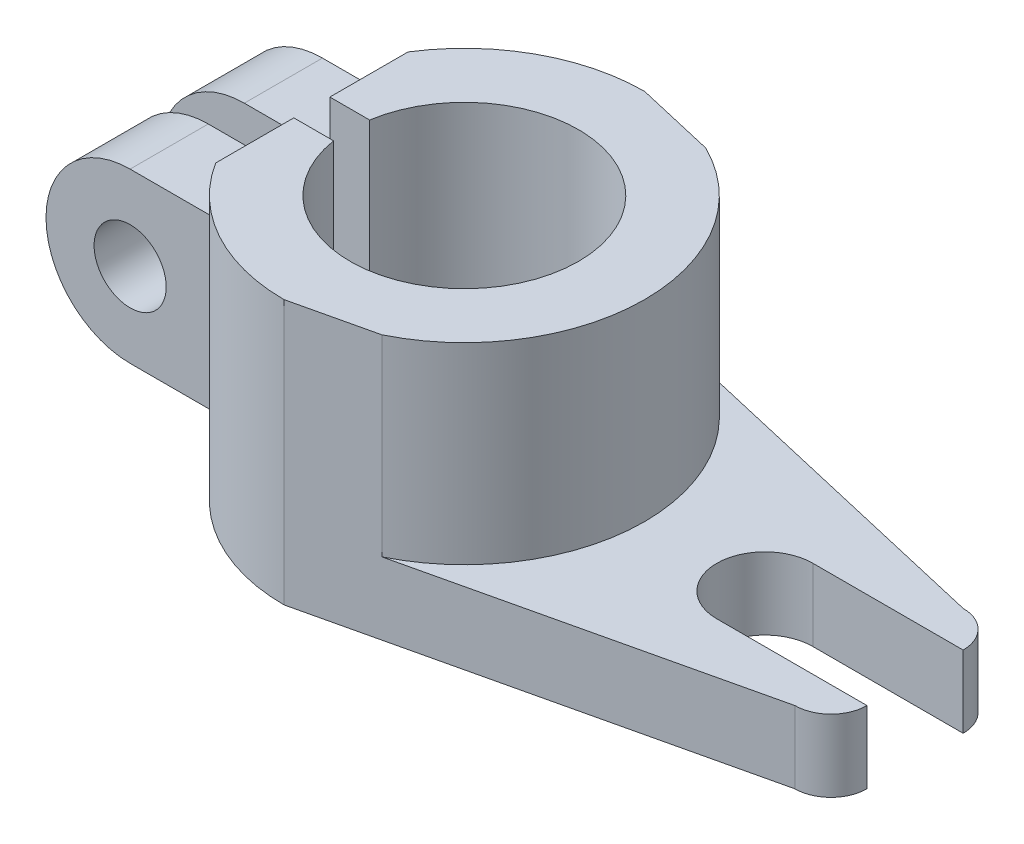
ISO-10303-21;
HEADER;
FILE_DESCRIPTION(('STEP AP214'),'2;1');
FILE_NAME('part.step','',(''),(''),'','','');
FILE_SCHEMA(('AUTOMOTIVE_DESIGN { 1 0 10303 214 1 1 1 1 }'));
ENDSEC;
DATA;
#1=APPLICATION_CONTEXT('core data for automotive mechanical design processes');
#2=APPLICATION_PROTOCOL_DEFINITION('international standard','automotive_design',2000,#1);
#3=PRODUCT_CONTEXT('',#1,'mechanical');
#4=PRODUCT('Part','Part','',(#3));
#5=PRODUCT_RELATED_PRODUCT_CATEGORY('part','',(#4));
#6=PRODUCT_DEFINITION_FORMATION('','',#4);
#7=PRODUCT_DEFINITION_CONTEXT('part definition',#1,'design');
#8=PRODUCT_DEFINITION('design','',#6,#7);
#9=PRODUCT_DEFINITION_SHAPE('','',#8);
#10=(LENGTH_UNIT() NAMED_UNIT(*) SI_UNIT(.MILLI.,.METRE.));
#11=(NAMED_UNIT(*) PLANE_ANGLE_UNIT() SI_UNIT($,.RADIAN.));
#12=(NAMED_UNIT(*) SI_UNIT($,.STERADIAN.) SOLID_ANGLE_UNIT());
#13=UNCERTAINTY_MEASURE_WITH_UNIT(LENGTH_MEASURE(1.E-05),#10,'distance_accuracy_value','');
#14=(GEOMETRIC_REPRESENTATION_CONTEXT(3) GLOBAL_UNCERTAINTY_ASSIGNED_CONTEXT((#13)) GLOBAL_UNIT_ASSIGNED_CONTEXT((#10,
#11,#12)) REPRESENTATION_CONTEXT('',''));
#15=CARTESIAN_POINT('',(0.,0.,0.));
#16=DIRECTION('',(0.,0.,1.));
#17=DIRECTION('',(1.,0.,0.));
#18=AXIS2_PLACEMENT_3D('',#15,#16,#17);
#19=CARTESIAN_POINT('',(-39.6122656575528,22.,-16.));
#20=DIRECTION('',(0.,0.,1.));
#21=DIRECTION('',(1.,0.,0.));
#22=AXIS2_PLACEMENT_3D('',#19,#20,#21);
#23=CYLINDRICAL_SURFACE('',#22,14.);
#24=DIRECTION('',(0.,0.,1.));
#25=VECTOR('',#24,1.);
#26=CARTESIAN_POINT('',(-39.6122656575528,36.,-16.));
#27=LINE('',#26,#25);
#28=CARTESIAN_POINT('',(-39.6122656575528,36.,3.));
#29=VERTEX_POINT('',#28);
#30=CARTESIAN_POINT('',(-39.6122656575528,36.,16.));
#31=VERTEX_POINT('',#30);
#32=EDGE_CURVE('E333',#29,#31,#27,.T.);
#33=ORIENTED_EDGE('',*,*,#32,.F.);
#34=CARTESIAN_POINT('',(-39.6122656575528,22.,3.));
#35=DIRECTION('',(0.,0.,1.));
#36=DIRECTION('',(1.,0.,0.));
#37=AXIS2_PLACEMENT_3D('',#34,#35,#36);
#38=CIRCLE('',#37,14.);
#39=CARTESIAN_POINT('',(-39.6122656575528,8.,3.));
#40=VERTEX_POINT('',#39);
#41=EDGE_CURVE('E56',#40,#29,#38,.F.);
#42=ORIENTED_EDGE('',*,*,#41,.F.);
#43=DIRECTION('',(0.,0.,1.));
#44=VECTOR('',#43,1.);
#45=CARTESIAN_POINT('',(-39.6122656575528,8.,-16.));
#46=LINE('',#45,#44);
#47=CARTESIAN_POINT('',(-39.6122656575528,8.,16.));
#48=VERTEX_POINT('',#47);
#49=EDGE_CURVE('E336',#40,#48,#46,.T.);
#50=ORIENTED_EDGE('',*,*,#49,.T.);
#51=CARTESIAN_POINT('',(-39.6122656575528,22.,16.));
#52=DIRECTION('',(0.,0.,1.));
#53=DIRECTION('',(1.,0.,0.));
#54=AXIS2_PLACEMENT_3D('',#51,#52,#53);
#55=CIRCLE('',#54,14.);
#56=EDGE_CURVE('E329',#31,#48,#55,.T.);
#57=ORIENTED_EDGE('',*,*,#56,.F.);
#58=EDGE_LOOP('',(#33,#42,#50,#57));
#59=FACE_BOUND('',#58,.T.);
#60=ADVANCED_FACE('F43',(#59),#23,.T.);
#61=CARTESIAN_POINT('',(-39.6122656575528,22.,-3.));
#62=DIRECTION('',(0.,0.,1.));
#63=DIRECTION('',(1.,0.,0.));
#64=AXIS2_PLACEMENT_3D('',#61,#62,#63);
#65=CIRCLE('',#64,14.);
#66=CARTESIAN_POINT('',(-39.6122656575528,8.,-3.));
#67=VERTEX_POINT('',#66);
#68=CARTESIAN_POINT('',(-39.6122656575528,36.,-3.));
#69=VERTEX_POINT('',#68);
#70=EDGE_CURVE('E453',#67,#69,#65,.F.);
#71=ORIENTED_EDGE('',*,*,#70,.T.);
#72=CARTESIAN_POINT('',(-39.6122656575528,36.,-16.));
#73=VERTEX_POINT('',#72);
#74=EDGE_CURVE('E294',#73,#69,#27,.T.);
#75=ORIENTED_EDGE('',*,*,#74,.F.);
#76=CARTESIAN_POINT('',(-39.6122656575528,22.,-16.));
#77=DIRECTION('',(0.,0.,1.));
#78=DIRECTION('',(1.,0.,0.));
#79=AXIS2_PLACEMENT_3D('',#76,#77,#78);
#80=CIRCLE('',#79,14.);
#81=CARTESIAN_POINT('',(-39.6122656575528,8.,-16.));
#82=VERTEX_POINT('',#81);
#83=EDGE_CURVE('E326',#73,#82,#80,.T.);
#84=ORIENTED_EDGE('',*,*,#83,.T.);
#85=EDGE_CURVE('E332',#82,#67,#46,.T.);
#86=ORIENTED_EDGE('',*,*,#85,.T.);
#87=EDGE_LOOP('',(#71,#75,#84,#86));
#88=FACE_BOUND('',#87,.T.);
#89=ADVANCED_FACE('F460',(#88),#23,.T.);
#90=CARTESIAN_POINT('',(-39.6122656575528,22.,-22.0274259538665));
#91=DIRECTION('',(0.,0.,1.));
#92=DIRECTION('',(1.,0.,0.));
#93=AXIS2_PLACEMENT_3D('',#90,#91,#92);
#94=CYLINDRICAL_SURFACE('',#93,6.);
#95=CARTESIAN_POINT('',(-39.6122656575528,22.,-16.));
#96=DIRECTION('',(0.,0.,-1.));
#97=DIRECTION('',(-1.,0.,0.));
#98=AXIS2_PLACEMENT_3D('',#95,#96,#97);
#99=CIRCLE('',#98,6.);
#100=CARTESIAN_POINT('',(-45.6122656575528,22.,-16.));
#101=VERTEX_POINT('',#100);
#102=EDGE_CURVE('E50',#101,#101,#99,.T.);
#103=ORIENTED_EDGE('',*,*,#102,.T.);
#104=EDGE_LOOP('',(#103));
#105=FACE_BOUND('',#104,.T.);
#106=CARTESIAN_POINT('',(-39.6122656575528,22.,-3.));
#107=DIRECTION('',(0.,0.,1.));
#108=DIRECTION('',(1.,0.,0.));
#109=AXIS2_PLACEMENT_3D('',#106,#107,#108);
#110=CIRCLE('',#109,6.);
#111=CARTESIAN_POINT('',(-33.6122656575528,22.,-3.));
#112=VERTEX_POINT('',#111);
#113=EDGE_CURVE('E454',#112,#112,#110,.F.);
#114=ORIENTED_EDGE('',*,*,#113,.F.);
#115=EDGE_LOOP('',(#114));
#116=FACE_BOUND('',#115,.T.);
#117=ADVANCED_FACE('F476',(#105,#116),#94,.F.);
#118=CARTESIAN_POINT('',(0.,8.,-16.));
#119=DIRECTION('',(0.,1.,0.));
#120=DIRECTION('',(0.,0.,1.));
#121=AXIS2_PLACEMENT_3D('',#118,#119,#120);
#122=PLANE('',#121);
#123=DIRECTION('',(1.,0.,0.));
#124=VECTOR('',#123,1.);
#125=CARTESIAN_POINT('',(0.,8.,-3.));
#126=LINE('',#125,#124);
#127=CARTESIAN_POINT('',(-25.377155080899,8.,-3.));
#128=VERTEX_POINT('',#127);
#129=EDGE_CURVE('E296',#67,#128,#126,.T.);
#130=ORIENTED_EDGE('',*,*,#129,.F.);
#131=ORIENTED_EDGE('',*,*,#85,.F.);
#132=DIRECTION('',(-1.,0.,0.));
#133=VECTOR('',#132,1.);
#134=CARTESIAN_POINT('',(0.,8.,-16.));
#135=LINE('',#134,#133);
#136=CARTESIAN_POINT('',(-25.377155080899,8.,-16.));
#137=VERTEX_POINT('',#136);
#138=EDGE_CURVE('E422',#137,#82,#135,.T.);
#139=ORIENTED_EDGE('',*,*,#138,.F.);
#140=DIRECTION('',(0.,0.,1.));
#141=VECTOR('',#140,1.);
#142=CARTESIAN_POINT('',(-25.377155080899,8.,-16.));
#143=LINE('',#142,#141);
#144=EDGE_CURVE('E424',#137,#128,#143,.T.);
#145=ORIENTED_EDGE('',*,*,#144,.T.);
#146=EDGE_LOOP('',(#130,#131,#139,#145));
#147=FACE_BOUND('',#146,.T.);
#148=ADVANCED_FACE('F463',(#147),#122,.F.);
#149=CARTESIAN_POINT('',(0.,36.,-16.));
#150=DIRECTION('',(0.,-1.,0.));
#151=DIRECTION('',(0.,0.,-1.));
#152=AXIS2_PLACEMENT_3D('',#149,#150,#151);
#153=PLANE('',#152);
#154=DIRECTION('',(-1.,0.,0.));
#155=VECTOR('',#154,1.);
#156=CARTESIAN_POINT('',(0.,36.,-3.));
#157=LINE('',#156,#155);
#158=CARTESIAN_POINT('',(-25.377155080899,36.,-3.));
#159=VERTEX_POINT('',#158);
#160=EDGE_CURVE('E286',#159,#69,#157,.T.);
#161=ORIENTED_EDGE('',*,*,#160,.F.);
#162=DIRECTION('',(0.,0.,1.));
#163=VECTOR('',#162,1.);
#164=CARTESIAN_POINT('',(-25.377155080899,36.,-16.));
#165=LINE('',#164,#163);
#166=CARTESIAN_POINT('',(-25.377155080899,36.,-16.));
#167=VERTEX_POINT('',#166);
#168=EDGE_CURVE('E292',#167,#159,#165,.T.);
#169=ORIENTED_EDGE('',*,*,#168,.F.);
#170=DIRECTION('',(1.,0.,0.));
#171=VECTOR('',#170,1.);
#172=CARTESIAN_POINT('',(0.,36.,-16.));
#173=LINE('',#172,#171);
#174=EDGE_CURVE('E443',#73,#167,#173,.T.);
#175=ORIENTED_EDGE('',*,*,#174,.F.);
#176=ORIENTED_EDGE('',*,*,#74,.T.);
#177=EDGE_LOOP('',(#161,#169,#175,#176));
#178=FACE_BOUND('',#177,.T.);
#179=ADVANCED_FACE('F289',(#178),#153,.F.);
#180=CARTESIAN_POINT('',(0.,44.,16.));
#181=DIRECTION('',(0.,0.,-1.));
#182=DIRECTION('',(-1.,0.,0.));
#183=AXIS2_PLACEMENT_3D('',#180,#181,#182);
#184=PLANE('',#183);
#185=CARTESIAN_POINT('',(-39.6122656575528,22.,16.));
#186=DIRECTION('',(0.,0.,1.));
#187=DIRECTION('',(1.,0.,0.));
#188=AXIS2_PLACEMENT_3D('',#185,#186,#187);
#189=CIRCLE('',#188,6.);
#190=CARTESIAN_POINT('',(-33.6122656575528,22.,16.));
#191=VERTEX_POINT('',#190);
#192=EDGE_CURVE('E340',#191,#191,#189,.T.);
#193=ORIENTED_EDGE('',*,*,#192,.F.);
#194=EDGE_LOOP('',(#193));
#195=FACE_BOUND('',#194,.T.);
#196=DIRECTION('',(1.,0.,0.));
#197=VECTOR('',#196,1.);
#198=CARTESIAN_POINT('',(0.,36.,16.));
#199=LINE('',#198,#197);
#200=CARTESIAN_POINT('',(-25.377155080899,36.,16.));
#201=VERTEX_POINT('',#200);
#202=EDGE_CURVE('E430',#31,#201,#199,.T.);
#203=ORIENTED_EDGE('',*,*,#202,.F.);
#204=ORIENTED_EDGE('',*,*,#56,.T.);
#205=DIRECTION('',(-1.,0.,0.));
#206=VECTOR('',#205,1.);
#207=CARTESIAN_POINT('',(0.,8.,16.));
#208=LINE('',#207,#206);
#209=CARTESIAN_POINT('',(-25.377155080899,8.,16.));
#210=VERTEX_POINT('',#209);
#211=EDGE_CURVE('E414',#210,#48,#208,.T.);
#212=ORIENTED_EDGE('',*,*,#211,.F.);
#213=DIRECTION('',(0.,-1.,0.));
#214=VECTOR('',#213,1.);
#215=CARTESIAN_POINT('',(-25.377155080899,44.,16.));
#216=LINE('',#215,#214);
#217=EDGE_CURVE('E345',#201,#210,#216,.T.);
#218=ORIENTED_EDGE('',*,*,#217,.F.);
#219=EDGE_LOOP('',(#203,#204,#212,#218));
#220=FACE_BOUND('',#219,.T.);
#221=ADVANCED_FACE('F482',(#195,#220),#184,.F.);
#222=CARTESIAN_POINT('',(0.,44.,-16.));
#223=DIRECTION('',(0.,0.,-1.));
#224=DIRECTION('',(-1.,0.,0.));
#225=AXIS2_PLACEMENT_3D('',#222,#223,#224);
#226=PLANE('',#225);
#227=ORIENTED_EDGE('',*,*,#102,.F.);
#228=EDGE_LOOP('',(#227));
#229=FACE_BOUND('',#228,.T.);
#230=ORIENTED_EDGE('',*,*,#83,.F.);
#231=ORIENTED_EDGE('',*,*,#174,.T.);
#232=DIRECTION('',(0.,-1.,0.));
#233=VECTOR('',#232,1.);
#234=CARTESIAN_POINT('',(-25.377155080899,44.,-16.));
#235=LINE('',#234,#233);
#236=EDGE_CURVE('E343',#167,#137,#235,.T.);
#237=ORIENTED_EDGE('',*,*,#236,.T.);
#238=ORIENTED_EDGE('',*,*,#138,.T.);
#239=EDGE_LOOP('',(#230,#231,#237,#238));
#240=FACE_BOUND('',#239,.T.);
#241=ADVANCED_FACE('F485',(#229,#240),#226,.T.);
#242=CARTESIAN_POINT('',(0.,44.,0.));
#243=DIRECTION('',(0.,-1.,0.));
#244=DIRECTION('',(0.,0.,-1.));
#245=AXIS2_PLACEMENT_3D('',#242,#243,#244);
#246=CYLINDRICAL_SURFACE('',#245,30.);
#247=CARTESIAN_POINT('',(-25.377155080899,44.,16.));
#248=VERTEX_POINT('',#247);
#249=EDGE_CURVE('E342',#248,#201,#216,.T.);
#250=ORIENTED_EDGE('',*,*,#249,.T.);
#251=ORIENTED_EDGE('',*,*,#217,.T.);
#252=DIRECTION('',(0.,1.,0.));
#253=VECTOR('',#252,1.);
#254=CARTESIAN_POINT('',(-25.377155080899,0.,16.));
#255=LINE('',#254,#253);
#256=CARTESIAN_POINT('',(-25.377155080899,0.,16.));
#257=VERTEX_POINT('',#256);
#258=EDGE_CURVE('E410',#257,#210,#255,.T.);
#259=ORIENTED_EDGE('',*,*,#258,.F.);
#260=CARTESIAN_POINT('',(0.,0.,0.));
#261=DIRECTION('',(0.,1.,0.));
#262=DIRECTION('',(0.,0.,1.));
#263=AXIS2_PLACEMENT_3D('',#260,#261,#262);
#264=CIRCLE('',#263,30.);
#265=CARTESIAN_POINT('',(0.,0.,30.));
#266=VERTEX_POINT('',#265);
#267=EDGE_CURVE('E351',#257,#266,#264,.T.);
#268=ORIENTED_EDGE('',*,*,#267,.T.);
#269=DIRECTION('',(0.,-1.,0.));
#270=VECTOR('',#269,1.);
#271=CARTESIAN_POINT('',(0.,44.,30.));
#272=LINE('',#271,#270);
#273=CARTESIAN_POINT('',(0.,44.,30.));
#274=VERTEX_POINT('',#273);
#275=EDGE_CURVE('E367',#274,#266,#272,.T.);
#276=ORIENTED_EDGE('',*,*,#275,.F.);
#277=CARTESIAN_POINT('',(0.,44.,0.));
#278=DIRECTION('',(0.,1.,0.));
#279=DIRECTION('',(0.,0.,1.));
#280=AXIS2_PLACEMENT_3D('',#277,#278,#279);
#281=CIRCLE('',#280,30.);
#282=EDGE_CURVE('E370',#248,#274,#281,.T.);
#283=ORIENTED_EDGE('',*,*,#282,.F.);
#284=EDGE_LOOP('',(#250,#251,#259,#268,#276,#283));
#285=FACE_BOUND('',#284,.T.);
#286=ADVANCED_FACE('F404',(#285),#246,.T.);
#287=CARTESIAN_POINT('',(6.60155471397249,12.,28.4692047040064));
#288=DIRECTION('',(-0.225890482018287,0.,-0.974152703703863));
#289=DIRECTION('',(-0.974152703703863,0.,0.225890482018287));
#290=AXIS2_PLACEMENT_3D('',#287,#288,#289);
#291=PLANE('',#290);
#292=DIRECTION('',(0.974152703703863,0.,-0.225890482018287));
#293=VECTOR('',#292,1.);
#294=CARTESIAN_POINT('',(6.60155471397249,0.,28.4692047040064));
#295=LINE('',#294,#293);
#296=CARTESIAN_POINT('',(69.,0.,14.));
#297=VERTEX_POINT('',#296);
#298=EDGE_CURVE('E144',#266,#297,#295,.T.);
#299=ORIENTED_EDGE('',*,*,#298,.T.);
#300=DIRECTION('',(0.,-1.,0.));
#301=VECTOR('',#300,1.);
#302=CARTESIAN_POINT('',(69.,12.,14.));
#303=LINE('',#302,#301);
#304=CARTESIAN_POINT('',(69.,12.,14.));
#305=VERTEX_POINT('',#304);
#306=EDGE_CURVE('E11',#305,#297,#303,.T.);
#307=ORIENTED_EDGE('',*,*,#306,.F.);
#308=DIRECTION('',(0.974152703703863,0.,-0.225890482018287));
#309=VECTOR('',#308,1.);
#310=CARTESIAN_POINT('',(6.60155471397249,12.,28.4692047040064));
#311=LINE('',#310,#309);
#312=CARTESIAN_POINT('',(13.2031094279449,12.,26.9384094080128));
#313=VERTEX_POINT('',#312);
#314=EDGE_CURVE('E105',#313,#305,#311,.T.);
#315=ORIENTED_EDGE('',*,*,#314,.F.);
#316=DIRECTION('',(0.,-1.,0.));
#317=VECTOR('',#316,1.);
#318=CARTESIAN_POINT('',(13.2031094279449,44.,26.9384094080128));
#319=LINE('',#318,#317);
#320=CARTESIAN_POINT('',(13.2031094279449,44.,26.9384094080128));
#321=VERTEX_POINT('',#320);
#322=EDGE_CURVE('E150',#321,#313,#319,.T.);
#323=ORIENTED_EDGE('',*,*,#322,.F.);
#324=DIRECTION('',(0.974152703703863,0.,-0.225890482018287));
#325=VECTOR('',#324,1.);
#326=CARTESIAN_POINT('',(6.60155471397249,44.,28.4692047040064));
#327=LINE('',#326,#325);
#328=EDGE_CURVE('E346',#274,#321,#327,.T.);
#329=ORIENTED_EDGE('',*,*,#328,.F.);
#330=ORIENTED_EDGE('',*,*,#275,.T.);
#331=EDGE_LOOP('',(#299,#307,#315,#323,#329,#330));
#332=FACE_BOUND('',#331,.T.);
#333=ADVANCED_FACE('F44',(#332),#291,.F.);
#334=CARTESIAN_POINT('',(69.,12.,8.00000000000001));
#335=DIRECTION('',(0.,-1.,0.));
#336=DIRECTION('',(0.,0.,-1.));
#337=AXIS2_PLACEMENT_3D('',#334,#335,#336);
#338=CYLINDRICAL_SURFACE('',#337,6.);
#339=CARTESIAN_POINT('',(69.,0.,8.00000000000001));
#340=DIRECTION('',(0.,1.,0.));
#341=DIRECTION('',(0.,0.,1.));
#342=AXIS2_PLACEMENT_3D('',#339,#340,#341);
#343=CIRCLE('',#342,6.);
#344=CARTESIAN_POINT('',(75.,0.,8.00000000000001));
#345=VERTEX_POINT('',#344);
#346=EDGE_CURVE('E146',#345,#297,#343,.F.);
#347=ORIENTED_EDGE('',*,*,#346,.F.);
#348=DIRECTION('',(0.,-1.,0.));
#349=VECTOR('',#348,1.);
#350=CARTESIAN_POINT('',(75.,12.,8.00000000000001));
#351=LINE('',#350,#349);
#352=CARTESIAN_POINT('',(75.,12.,8.00000000000001));
#353=VERTEX_POINT('',#352);
#354=EDGE_CURVE('E55',#353,#345,#351,.T.);
#355=ORIENTED_EDGE('',*,*,#354,.F.);
#356=CARTESIAN_POINT('',(69.,12.,8.00000000000001));
#357=DIRECTION('',(0.,1.,0.));
#358=DIRECTION('',(0.,0.,1.));
#359=AXIS2_PLACEMENT_3D('',#356,#357,#358);
#360=CIRCLE('',#359,6.);
#361=EDGE_CURVE('E140',#353,#305,#360,.F.);
#362=ORIENTED_EDGE('',*,*,#361,.T.);
#363=ORIENTED_EDGE('',*,*,#306,.T.);
#364=EDGE_LOOP('',(#347,#355,#362,#363));
#365=FACE_BOUND('',#364,.T.);
#366=ADVANCED_FACE('F175',(#365),#338,.T.);
#367=CARTESIAN_POINT('',(0.,12.,8.00000000000001));
#368=DIRECTION('',(0.,0.,-1.));
#369=DIRECTION('',(-1.,0.,0.));
#370=AXIS2_PLACEMENT_3D('',#367,#368,#369);
#371=PLANE('',#370);
#372=DIRECTION('',(1.,0.,0.));
#373=VECTOR('',#372,1.);
#374=CARTESIAN_POINT('',(0.,0.,8.00000000000001));
#375=LINE('',#374,#373);
#376=CARTESIAN_POINT('',(50.,0.,8.00000000000001));
#377=VERTEX_POINT('',#376);
#378=EDGE_CURVE('E152',#377,#345,#375,.T.);
#379=ORIENTED_EDGE('',*,*,#378,.F.);
#380=DIRECTION('',(0.,-1.,0.));
#381=VECTOR('',#380,1.);
#382=CARTESIAN_POINT('',(50.,12.,8.00000000000001));
#383=LINE('',#382,#381);
#384=CARTESIAN_POINT('',(50.,12.,8.00000000000001));
#385=VERTEX_POINT('',#384);
#386=EDGE_CURVE('E121',#385,#377,#383,.T.);
#387=ORIENTED_EDGE('',*,*,#386,.F.);
#388=DIRECTION('',(1.,0.,0.));
#389=VECTOR('',#388,1.);
#390=CARTESIAN_POINT('',(0.,12.,8.00000000000001));
#391=LINE('',#390,#389);
#392=EDGE_CURVE('E133',#385,#353,#391,.T.);
#393=ORIENTED_EDGE('',*,*,#392,.T.);
#394=ORIENTED_EDGE('',*,*,#354,.T.);
#395=EDGE_LOOP('',(#379,#387,#393,#394));
#396=FACE_BOUND('',#395,.T.);
#397=ADVANCED_FACE('F169',(#396),#371,.T.);
#398=CARTESIAN_POINT('',(50.,12.,0.));
#399=DIRECTION('',(0.,-1.,0.));
#400=DIRECTION('',(0.,0.,-1.));
#401=AXIS2_PLACEMENT_3D('',#398,#399,#400);
#402=CYLINDRICAL_SURFACE('',#401,8.00000000000001);
#403=CARTESIAN_POINT('',(50.,0.,0.));
#404=DIRECTION('',(0.,1.,0.));
#405=DIRECTION('',(0.,0.,1.));
#406=AXIS2_PLACEMENT_3D('',#403,#404,#405);
#407=CIRCLE('',#406,8.00000000000001);
#408=CARTESIAN_POINT('',(50.,0.,-8.00000000000001));
#409=VERTEX_POINT('',#408);
#410=EDGE_CURVE('E122',#409,#377,#407,.T.);
#411=ORIENTED_EDGE('',*,*,#410,.F.);
#412=DIRECTION('',(0.,-1.,0.));
#413=VECTOR('',#412,1.);
#414=CARTESIAN_POINT('',(50.,12.,-8.00000000000001));
#415=LINE('',#414,#413);
#416=CARTESIAN_POINT('',(50.,12.,-8.00000000000001));
#417=VERTEX_POINT('',#416);
#418=EDGE_CURVE('E114',#417,#409,#415,.T.);
#419=ORIENTED_EDGE('',*,*,#418,.F.);
#420=CARTESIAN_POINT('',(50.,12.,0.));
#421=DIRECTION('',(0.,1.,0.));
#422=DIRECTION('',(0.,0.,1.));
#423=AXIS2_PLACEMENT_3D('',#420,#421,#422);
#424=CIRCLE('',#423,8.00000000000001);
#425=EDGE_CURVE('E118',#417,#385,#424,.T.);
#426=ORIENTED_EDGE('',*,*,#425,.T.);
#427=ORIENTED_EDGE('',*,*,#386,.T.);
#428=EDGE_LOOP('',(#411,#419,#426,#427));
#429=FACE_BOUND('',#428,.T.);
#430=ADVANCED_FACE('F120',(#429),#402,.F.);
#431=CARTESIAN_POINT('',(0.,12.,-8.00000000000001));
#432=DIRECTION('',(0.,0.,-1.));
#433=DIRECTION('',(-1.,0.,0.));
#434=AXIS2_PLACEMENT_3D('',#431,#432,#433);
#435=PLANE('',#434);
#436=DIRECTION('',(1.,0.,0.));
#437=VECTOR('',#436,1.);
#438=CARTESIAN_POINT('',(0.,0.,-8.00000000000001));
#439=LINE('',#438,#437);
#440=CARTESIAN_POINT('',(75.,0.,-8.00000000000001));
#441=VERTEX_POINT('',#440);
#442=EDGE_CURVE('E153',#409,#441,#439,.T.);
#443=ORIENTED_EDGE('',*,*,#442,.T.);
#444=DIRECTION('',(0.,-1.,0.));
#445=VECTOR('',#444,1.);
#446=CARTESIAN_POINT('',(75.,12.,-8.00000000000001));
#447=LINE('',#446,#445);
#448=CARTESIAN_POINT('',(75.,12.,-8.00000000000001));
#449=VERTEX_POINT('',#448);
#450=EDGE_CURVE('E123',#449,#441,#447,.T.);
#451=ORIENTED_EDGE('',*,*,#450,.F.);
#452=DIRECTION('',(1.,0.,0.));
#453=VECTOR('',#452,1.);
#454=CARTESIAN_POINT('',(0.,12.,-8.00000000000001));
#455=LINE('',#454,#453);
#456=EDGE_CURVE('E130',#417,#449,#455,.T.);
#457=ORIENTED_EDGE('',*,*,#456,.F.);
#458=ORIENTED_EDGE('',*,*,#418,.T.);
#459=EDGE_LOOP('',(#443,#451,#457,#458));
#460=FACE_BOUND('',#459,.T.);
#461=ADVANCED_FACE('F128',(#460),#435,.F.);
#462=CARTESIAN_POINT('',(69.,12.,-8.00000000000001));
#463=DIRECTION('',(0.,-1.,0.));
#464=DIRECTION('',(0.,0.,-1.));
#465=AXIS2_PLACEMENT_3D('',#462,#463,#464);
#466=CYLINDRICAL_SURFACE('',#465,6.);
#467=CARTESIAN_POINT('',(69.,0.,-8.00000000000001));
#468=DIRECTION('',(0.,1.,0.));
#469=DIRECTION('',(0.,0.,1.));
#470=AXIS2_PLACEMENT_3D('',#467,#468,#469);
#471=CIRCLE('',#470,6.);
#472=CARTESIAN_POINT('',(69.,0.,-14.));
#473=VERTEX_POINT('',#472);
#474=EDGE_CURVE('E160',#441,#473,#471,.T.);
#475=ORIENTED_EDGE('',*,*,#474,.T.);
#476=DIRECTION('',(0.,-1.,0.));
#477=VECTOR('',#476,1.);
#478=CARTESIAN_POINT('',(69.,12.,-14.));
#479=LINE('',#478,#477);
#480=CARTESIAN_POINT('',(69.,12.,-14.));
#481=VERTEX_POINT('',#480);
#482=EDGE_CURVE('E92',#481,#473,#479,.T.);
#483=ORIENTED_EDGE('',*,*,#482,.F.);
#484=CARTESIAN_POINT('',(69.,12.,-8.00000000000001));
#485=DIRECTION('',(0.,1.,0.));
#486=DIRECTION('',(0.,0.,1.));
#487=AXIS2_PLACEMENT_3D('',#484,#485,#486);
#488=CIRCLE('',#487,6.);
#489=EDGE_CURVE('E69',#449,#481,#488,.T.);
#490=ORIENTED_EDGE('',*,*,#489,.F.);
#491=ORIENTED_EDGE('',*,*,#450,.T.);
#492=EDGE_LOOP('',(#475,#483,#490,#491));
#493=FACE_BOUND('',#492,.T.);
#494=ADVANCED_FACE('F177',(#493),#466,.T.);
#495=CARTESIAN_POINT('',(6.60155471397249,12.,-28.4692047040064));
#496=DIRECTION('',(0.225890482018287,0.,-0.974152703703863));
#497=DIRECTION('',(-0.974152703703863,0.,-0.225890482018287));
#498=AXIS2_PLACEMENT_3D('',#495,#496,#497);
#499=PLANE('',#498);
#500=DIRECTION('',(0.974152703703863,0.,0.225890482018287));
#501=VECTOR('',#500,1.);
#502=CARTESIAN_POINT('',(6.60155471397249,0.,-28.4692047040064));
#503=LINE('',#502,#501);
#504=CARTESIAN_POINT('',(0.,0.,-30.));
#505=VERTEX_POINT('',#504);
#506=EDGE_CURVE('E157',#505,#473,#503,.T.);
#507=ORIENTED_EDGE('',*,*,#506,.F.);
#508=DIRECTION('',(0.,-1.,0.));
#509=VECTOR('',#508,1.);
#510=CARTESIAN_POINT('',(0.,44.,-30.));
#511=LINE('',#510,#509);
#512=CARTESIAN_POINT('',(0.,44.,-30.));
#513=VERTEX_POINT('',#512);
#514=EDGE_CURVE('E390',#513,#505,#511,.T.);
#515=ORIENTED_EDGE('',*,*,#514,.F.);
#516=DIRECTION('',(0.974152703703863,0.,0.225890482018287));
#517=VECTOR('',#516,1.);
#518=CARTESIAN_POINT('',(6.60155471397249,44.,-28.4692047040064));
#519=LINE('',#518,#517);
#520=CARTESIAN_POINT('',(13.2031094279449,44.,-26.9384094080128));
#521=VERTEX_POINT('',#520);
#522=EDGE_CURVE('E354',#513,#521,#519,.T.);
#523=ORIENTED_EDGE('',*,*,#522,.T.);
#524=DIRECTION('',(0.,-1.,0.));
#525=VECTOR('',#524,1.);
#526=CARTESIAN_POINT('',(13.2031094279449,44.,-26.9384094080128));
#527=LINE('',#526,#525);
#528=CARTESIAN_POINT('',(13.2031094279449,12.,-26.9384094080128));
#529=VERTEX_POINT('',#528);
#530=EDGE_CURVE('E184',#521,#529,#527,.T.);
#531=ORIENTED_EDGE('',*,*,#530,.T.);
#532=DIRECTION('',(0.974152703703863,0.,0.225890482018287));
#533=VECTOR('',#532,1.);
#534=CARTESIAN_POINT('',(6.60155471397249,12.,-28.4692047040064));
#535=LINE('',#534,#533);
#536=EDGE_CURVE('E145',#529,#481,#535,.T.);
#537=ORIENTED_EDGE('',*,*,#536,.T.);
#538=ORIENTED_EDGE('',*,*,#482,.T.);
#539=EDGE_LOOP('',(#507,#515,#523,#531,#537,#538));
#540=FACE_BOUND('',#539,.T.);
#541=ADVANCED_FACE('F181',(#540),#499,.T.);
#542=CARTESIAN_POINT('',(0.,12.,0.));
#543=DIRECTION('',(0.,1.,0.));
#544=DIRECTION('',(0.,0.,1.));
#545=AXIS2_PLACEMENT_3D('',#542,#543,#544);
#546=PLANE('',#545);
#547=CARTESIAN_POINT('',(0.,12.,0.));
#548=DIRECTION('',(0.,1.,0.));
#549=DIRECTION('',(0.,0.,1.));
#550=AXIS2_PLACEMENT_3D('',#547,#548,#549);
#551=CIRCLE('',#550,30.);
#552=EDGE_CURVE('E162',#313,#529,#551,.T.);
#553=ORIENTED_EDGE('',*,*,#552,.F.);
#554=ORIENTED_EDGE('',*,*,#314,.T.);
#555=ORIENTED_EDGE('',*,*,#361,.F.);
#556=ORIENTED_EDGE('',*,*,#392,.F.);
#557=ORIENTED_EDGE('',*,*,#425,.F.);
#558=ORIENTED_EDGE('',*,*,#456,.T.);
#559=ORIENTED_EDGE('',*,*,#489,.T.);
#560=ORIENTED_EDGE('',*,*,#536,.F.);
#561=EDGE_LOOP('',(#553,#554,#555,#556,#557,#558,#559,#560));
#562=FACE_BOUND('',#561,.T.);
#563=ADVANCED_FACE('F134',(#562),#546,.T.);
#564=CARTESIAN_POINT('',(0.,0.,0.));
#565=DIRECTION('',(0.,1.,0.));
#566=DIRECTION('',(0.,0.,1.));
#567=AXIS2_PLACEMENT_3D('',#564,#565,#566);
#568=PLANE('',#567);
#569=ORIENTED_EDGE('',*,*,#267,.F.);
#570=DIRECTION('',(0.,0.,1.));
#571=VECTOR('',#570,1.);
#572=CARTESIAN_POINT('',(-25.377155080899,0.,-16.));
#573=LINE('',#572,#571);
#574=CARTESIAN_POINT('',(-25.377155080899,0.,3.));
#575=VERTEX_POINT('',#574);
#576=EDGE_CURVE('E402',#575,#257,#573,.T.);
#577=ORIENTED_EDGE('',*,*,#576,.F.);
#578=DIRECTION('',(-1.,0.,0.));
#579=VECTOR('',#578,1.);
#580=CARTESIAN_POINT('',(0.,0.,3.));
#581=LINE('',#580,#579);
#582=CARTESIAN_POINT('',(-18.7616630392937,0.,3.));
#583=VERTEX_POINT('',#582);
#584=EDGE_CURVE('E377',#583,#575,#581,.T.);
#585=ORIENTED_EDGE('',*,*,#584,.F.);
#586=CARTESIAN_POINT('',(0.,0.,0.));
#587=DIRECTION('',(0.,1.,0.));
#588=DIRECTION('',(0.,0.,1.));
#589=AXIS2_PLACEMENT_3D('',#586,#587,#588);
#590=CIRCLE('',#589,19.);
#591=CARTESIAN_POINT('',(-18.7616630392937,0.,-3.));
#592=VERTEX_POINT('',#591);
#593=EDGE_CURVE('E374',#583,#592,#590,.T.);
#594=ORIENTED_EDGE('',*,*,#593,.T.);
#595=DIRECTION('',(-1.,0.,0.));
#596=VECTOR('',#595,1.);
#597=CARTESIAN_POINT('',(0.,0.,-3.));
#598=LINE('',#597,#596);
#599=CARTESIAN_POINT('',(-25.377155080899,0.,-3.));
#600=VERTEX_POINT('',#599);
#601=EDGE_CURVE('E375',#592,#600,#598,.T.);
#602=ORIENTED_EDGE('',*,*,#601,.T.);
#603=CARTESIAN_POINT('',(-25.377155080899,0.,-16.));
#604=VERTEX_POINT('',#603);
#605=EDGE_CURVE('E429',#604,#600,#573,.T.);
#606=ORIENTED_EDGE('',*,*,#605,.F.);
#607=CARTESIAN_POINT('',(0.,0.,0.));
#608=DIRECTION('',(0.,1.,0.));
#609=DIRECTION('',(0.,0.,1.));
#610=AXIS2_PLACEMENT_3D('',#607,#608,#609);
#611=CIRCLE('',#610,30.);
#612=EDGE_CURVE('E349',#505,#604,#611,.T.);
#613=ORIENTED_EDGE('',*,*,#612,.F.);
#614=ORIENTED_EDGE('',*,*,#506,.T.);
#615=ORIENTED_EDGE('',*,*,#474,.F.);
#616=ORIENTED_EDGE('',*,*,#442,.F.);
#617=ORIENTED_EDGE('',*,*,#410,.T.);
#618=ORIENTED_EDGE('',*,*,#378,.T.);
#619=ORIENTED_EDGE('',*,*,#346,.T.);
#620=ORIENTED_EDGE('',*,*,#298,.F.);
#621=EDGE_LOOP('',(#569,#577,#585,#594,#602,#606,#613,#614,#615,#616,#617,#618,#619,#620));
#622=FACE_BOUND('',#621,.T.);
#623=ADVANCED_FACE('F176',(#622),#568,.F.);
#624=CARTESIAN_POINT('',(0.,44.,0.));
#625=DIRECTION('',(0.,-1.,0.));
#626=DIRECTION('',(0.,0.,-1.));
#627=AXIS2_PLACEMENT_3D('',#624,#625,#626);
#628=CYLINDRICAL_SURFACE('',#627,30.);
#629=ORIENTED_EDGE('',*,*,#552,.T.);
#630=ORIENTED_EDGE('',*,*,#530,.F.);
#631=CARTESIAN_POINT('',(0.,44.,0.));
#632=DIRECTION('',(0.,1.,0.));
#633=DIRECTION('',(0.,0.,1.));
#634=AXIS2_PLACEMENT_3D('',#631,#632,#633);
#635=CIRCLE('',#634,30.);
#636=EDGE_CURVE('E355',#321,#521,#635,.T.);
#637=ORIENTED_EDGE('',*,*,#636,.F.);
#638=ORIENTED_EDGE('',*,*,#322,.T.);
#639=EDGE_LOOP('',(#629,#630,#637,#638));
#640=FACE_BOUND('',#639,.T.);
#641=ADVANCED_FACE('F393',(#640),#628,.T.);
#642=CARTESIAN_POINT('',(0.,44.,0.));
#643=DIRECTION('',(0.,-1.,0.));
#644=DIRECTION('',(0.,0.,-1.));
#645=AXIS2_PLACEMENT_3D('',#642,#643,#644);
#646=CYLINDRICAL_SURFACE('',#645,30.);
#647=ORIENTED_EDGE('',*,*,#612,.T.);
#648=DIRECTION('',(0.,1.,0.));
#649=VECTOR('',#648,1.);
#650=CARTESIAN_POINT('',(-25.377155080899,0.,-16.));
#651=LINE('',#650,#649);
#652=EDGE_CURVE('E420',#604,#137,#651,.T.);
#653=ORIENTED_EDGE('',*,*,#652,.T.);
#654=ORIENTED_EDGE('',*,*,#236,.F.);
#655=CARTESIAN_POINT('',(-25.377155080899,44.,-16.));
#656=VERTEX_POINT('',#655);
#657=EDGE_CURVE('E304',#656,#167,#235,.T.);
#658=ORIENTED_EDGE('',*,*,#657,.F.);
#659=CARTESIAN_POINT('',(0.,44.,0.));
#660=DIRECTION('',(0.,1.,0.));
#661=DIRECTION('',(0.,0.,1.));
#662=AXIS2_PLACEMENT_3D('',#659,#660,#661);
#663=CIRCLE('',#662,30.);
#664=EDGE_CURVE('E357',#513,#656,#663,.T.);
#665=ORIENTED_EDGE('',*,*,#664,.F.);
#666=ORIENTED_EDGE('',*,*,#514,.T.);
#667=EDGE_LOOP('',(#647,#653,#654,#658,#665,#666));
#668=FACE_BOUND('',#667,.T.);
#669=ADVANCED_FACE('F472',(#668),#646,.T.);
#670=CARTESIAN_POINT('',(0.,44.,-3.));
#671=DIRECTION('',(0.,0.,1.));
#672=DIRECTION('',(1.,0.,0.));
#673=AXIS2_PLACEMENT_3D('',#670,#671,#672);
#674=PLANE('',#673);
#675=DIRECTION('',(0.,1.,0.));
#676=VECTOR('',#675,1.);
#677=CARTESIAN_POINT('',(-25.377155080899,44.,-3.));
#678=LINE('',#677,#676);
#679=CARTESIAN_POINT('',(-25.377155080899,44.,-3.));
#680=VERTEX_POINT('',#679);
#681=EDGE_CURVE('E305',#159,#680,#678,.T.);
#682=ORIENTED_EDGE('',*,*,#681,.F.);
#683=ORIENTED_EDGE('',*,*,#160,.T.);
#684=ORIENTED_EDGE('',*,*,#70,.F.);
#685=ORIENTED_EDGE('',*,*,#129,.T.);
#686=DIRECTION('',(0.,1.,0.));
#687=VECTOR('',#686,1.);
#688=CARTESIAN_POINT('',(-25.377155080899,44.,-3.));
#689=LINE('',#688,#687);
#690=EDGE_CURVE('E316',#600,#128,#689,.T.);
#691=ORIENTED_EDGE('',*,*,#690,.F.);
#692=ORIENTED_EDGE('',*,*,#601,.F.);
#693=DIRECTION('',(0.,-1.,0.));
#694=VECTOR('',#693,1.);
#695=CARTESIAN_POINT('',(-18.7616630392937,44.,-3.));
#696=LINE('',#695,#694);
#697=CARTESIAN_POINT('',(-18.7616630392937,44.,-3.));
#698=VERTEX_POINT('',#697);
#699=EDGE_CURVE('E389',#698,#592,#696,.T.);
#700=ORIENTED_EDGE('',*,*,#699,.F.);
#701=DIRECTION('',(-1.,0.,0.));
#702=VECTOR('',#701,1.);
#703=CARTESIAN_POINT('',(0.,44.,-3.));
#704=LINE('',#703,#702);
#705=EDGE_CURVE('E313',#698,#680,#704,.T.);
#706=ORIENTED_EDGE('',*,*,#705,.T.);
#707=EDGE_LOOP('',(#682,#683,#684,#685,#691,#692,#700,#706));
#708=FACE_BOUND('',#707,.T.);
#709=ORIENTED_EDGE('',*,*,#113,.T.);
#710=EDGE_LOOP('',(#709));
#711=FACE_BOUND('',#710,.T.);
#712=ADVANCED_FACE('F311',(#708,#711),#674,.T.);
#713=CARTESIAN_POINT('',(0.,44.,0.));
#714=DIRECTION('',(0.,-1.,0.));
#715=DIRECTION('',(0.,0.,-1.));
#716=AXIS2_PLACEMENT_3D('',#713,#714,#715);
#717=CYLINDRICAL_SURFACE('',#716,19.);
#718=ORIENTED_EDGE('',*,*,#593,.F.);
#719=DIRECTION('',(0.,-1.,0.));
#720=VECTOR('',#719,1.);
#721=CARTESIAN_POINT('',(-18.7616630392937,44.,3.));
#722=LINE('',#721,#720);
#723=CARTESIAN_POINT('',(-18.7616630392937,44.,3.));
#724=VERTEX_POINT('',#723);
#725=EDGE_CURVE('E381',#724,#583,#722,.T.);
#726=ORIENTED_EDGE('',*,*,#725,.F.);
#727=CARTESIAN_POINT('',(0.,44.,0.));
#728=DIRECTION('',(0.,1.,0.));
#729=DIRECTION('',(0.,0.,1.));
#730=AXIS2_PLACEMENT_3D('',#727,#728,#729);
#731=CIRCLE('',#730,19.);
#732=EDGE_CURVE('E363',#724,#698,#731,.T.);
#733=ORIENTED_EDGE('',*,*,#732,.T.);
#734=ORIENTED_EDGE('',*,*,#699,.T.);
#735=EDGE_LOOP('',(#718,#726,#733,#734));
#736=FACE_BOUND('',#735,.T.);
#737=ADVANCED_FACE('F470',(#736),#717,.F.);
#738=CARTESIAN_POINT('',(0.,44.,3.));
#739=DIRECTION('',(0.,0.,1.));
#740=DIRECTION('',(1.,0.,0.));
#741=AXIS2_PLACEMENT_3D('',#738,#739,#740);
#742=PLANE('',#741);
#743=DIRECTION('',(0.,1.,0.));
#744=VECTOR('',#743,1.);
#745=CARTESIAN_POINT('',(-25.377155080899,44.,3.));
#746=LINE('',#745,#744);
#747=CARTESIAN_POINT('',(-25.377155080899,8.,3.));
#748=VERTEX_POINT('',#747);
#749=EDGE_CURVE('E314',#575,#748,#746,.T.);
#750=ORIENTED_EDGE('',*,*,#749,.T.);
#751=DIRECTION('',(1.,0.,0.));
#752=VECTOR('',#751,1.);
#753=CARTESIAN_POINT('',(0.,8.,3.));
#754=LINE('',#753,#752);
#755=EDGE_CURVE('E447',#40,#748,#754,.T.);
#756=ORIENTED_EDGE('',*,*,#755,.F.);
#757=ORIENTED_EDGE('',*,*,#41,.T.);
#758=DIRECTION('',(-1.,0.,0.));
#759=VECTOR('',#758,1.);
#760=CARTESIAN_POINT('',(0.,36.,3.));
#761=LINE('',#760,#759);
#762=CARTESIAN_POINT('',(-25.377155080899,36.,3.));
#763=VERTEX_POINT('',#762);
#764=EDGE_CURVE('E449',#763,#29,#761,.T.);
#765=ORIENTED_EDGE('',*,*,#764,.F.);
#766=DIRECTION('',(0.,1.,0.));
#767=VECTOR('',#766,1.);
#768=CARTESIAN_POINT('',(-25.377155080899,44.,3.));
#769=LINE('',#768,#767);
#770=CARTESIAN_POINT('',(-25.377155080899,44.,3.));
#771=VERTEX_POINT('',#770);
#772=EDGE_CURVE('E317',#763,#771,#769,.T.);
#773=ORIENTED_EDGE('',*,*,#772,.T.);
#774=DIRECTION('',(-1.,0.,0.));
#775=VECTOR('',#774,1.);
#776=CARTESIAN_POINT('',(0.,44.,3.));
#777=LINE('',#776,#775);
#778=EDGE_CURVE('E364',#724,#771,#777,.T.);
#779=ORIENTED_EDGE('',*,*,#778,.F.);
#780=ORIENTED_EDGE('',*,*,#725,.T.);
#781=ORIENTED_EDGE('',*,*,#584,.T.);
#782=EDGE_LOOP('',(#750,#756,#757,#765,#773,#779,#780,#781));
#783=FACE_BOUND('',#782,.T.);
#784=CARTESIAN_POINT('',(-39.6122656575528,22.,3.));
#785=DIRECTION('',(0.,0.,1.));
#786=DIRECTION('',(1.,0.,0.));
#787=AXIS2_PLACEMENT_3D('',#784,#785,#786);
#788=CIRCLE('',#787,6.);
#789=CARTESIAN_POINT('',(-33.6122656575528,22.,3.));
#790=VERTEX_POINT('',#789);
#791=EDGE_CURVE('E411',#790,#790,#788,.F.);
#792=ORIENTED_EDGE('',*,*,#791,.F.);
#793=EDGE_LOOP('',(#792));
#794=FACE_BOUND('',#793,.T.);
#795=ADVANCED_FACE('F520',(#783,#794),#742,.F.);
#796=CARTESIAN_POINT('',(0.,44.,0.));
#797=DIRECTION('',(0.,1.,0.));
#798=DIRECTION('',(0.,0.,1.));
#799=AXIS2_PLACEMENT_3D('',#796,#797,#798);
#800=PLANE('',#799);
#801=DIRECTION('',(0.,0.,1.));
#802=VECTOR('',#801,1.);
#803=CARTESIAN_POINT('',(-25.377155080899,44.,-16.));
#804=LINE('',#803,#802);
#805=EDGE_CURVE('E310',#771,#248,#804,.T.);
#806=ORIENTED_EDGE('',*,*,#805,.T.);
#807=ORIENTED_EDGE('',*,*,#282,.T.);
#808=ORIENTED_EDGE('',*,*,#328,.T.);
#809=ORIENTED_EDGE('',*,*,#636,.T.);
#810=ORIENTED_EDGE('',*,*,#522,.F.);
#811=ORIENTED_EDGE('',*,*,#664,.T.);
#812=EDGE_CURVE('E321',#656,#680,#804,.T.);
#813=ORIENTED_EDGE('',*,*,#812,.T.);
#814=ORIENTED_EDGE('',*,*,#705,.F.);
#815=ORIENTED_EDGE('',*,*,#732,.F.);
#816=ORIENTED_EDGE('',*,*,#778,.T.);
#817=EDGE_LOOP('',(#806,#807,#808,#809,#810,#811,#813,#814,#815,#816));
#818=FACE_BOUND('',#817,.T.);
#819=ADVANCED_FACE('F471',(#818),#800,.T.);
#820=ORIENTED_EDGE('',*,*,#791,.T.);
#821=EDGE_LOOP('',(#820));
#822=FACE_BOUND('',#821,.T.);
#823=ORIENTED_EDGE('',*,*,#192,.T.);
#824=EDGE_LOOP('',(#823));
#825=FACE_BOUND('',#824,.T.);
#826=ADVANCED_FACE('F508',(#822,#825),#94,.F.);
#827=ORIENTED_EDGE('',*,*,#49,.F.);
#828=ORIENTED_EDGE('',*,*,#755,.T.);
#829=EDGE_CURVE('E426',#748,#210,#143,.T.);
#830=ORIENTED_EDGE('',*,*,#829,.T.);
#831=ORIENTED_EDGE('',*,*,#211,.T.);
#832=EDGE_LOOP('',(#827,#828,#830,#831));
#833=FACE_BOUND('',#832,.T.);
#834=ADVANCED_FACE('F502',(#833),#122,.F.);
#835=EDGE_CURVE('E308',#763,#201,#165,.T.);
#836=ORIENTED_EDGE('',*,*,#835,.F.);
#837=ORIENTED_EDGE('',*,*,#764,.T.);
#838=ORIENTED_EDGE('',*,*,#32,.T.);
#839=ORIENTED_EDGE('',*,*,#202,.T.);
#840=EDGE_LOOP('',(#836,#837,#838,#839));
#841=FACE_BOUND('',#840,.T.);
#842=ADVANCED_FACE('F506',(#841),#153,.F.);
#843=CARTESIAN_POINT('',(-25.377155080899,0.,-16.));
#844=DIRECTION('',(1.,0.,0.));
#845=DIRECTION('',(0.,0.,-1.));
#846=AXIS2_PLACEMENT_3D('',#843,#844,#845);
#847=PLANE('',#846);
#848=ORIENTED_EDGE('',*,*,#690,.T.);
#849=ORIENTED_EDGE('',*,*,#144,.F.);
#850=ORIENTED_EDGE('',*,*,#652,.F.);
#851=ORIENTED_EDGE('',*,*,#605,.T.);
#852=EDGE_LOOP('',(#848,#849,#850,#851));
#853=FACE_BOUND('',#852,.T.);
#854=ADVANCED_FACE('F465',(#853),#847,.F.);
#855=ORIENTED_EDGE('',*,*,#576,.T.);
#856=ORIENTED_EDGE('',*,*,#258,.T.);
#857=ORIENTED_EDGE('',*,*,#829,.F.);
#858=ORIENTED_EDGE('',*,*,#749,.F.);
#859=EDGE_LOOP('',(#855,#856,#857,#858));
#860=FACE_BOUND('',#859,.T.);
#861=ADVANCED_FACE('F818',(#860),#847,.F.);
#862=CARTESIAN_POINT('',(-25.377155080899,0.,-16.));
#863=DIRECTION('',(1.,0.,0.));
#864=DIRECTION('',(0.,0.,-1.));
#865=AXIS2_PLACEMENT_3D('',#862,#863,#864);
#866=PLANE('',#865);
#867=ORIENTED_EDGE('',*,*,#835,.T.);
#868=ORIENTED_EDGE('',*,*,#249,.F.);
#869=ORIENTED_EDGE('',*,*,#805,.F.);
#870=ORIENTED_EDGE('',*,*,#772,.F.);
#871=EDGE_LOOP('',(#867,#868,#869,#870));
#872=FACE_BOUND('',#871,.T.);
#873=ADVANCED_FACE('F823',(#872),#866,.F.);
#874=ORIENTED_EDGE('',*,*,#681,.T.);
#875=ORIENTED_EDGE('',*,*,#812,.F.);
#876=ORIENTED_EDGE('',*,*,#657,.T.);
#877=ORIENTED_EDGE('',*,*,#168,.T.);
#878=EDGE_LOOP('',(#874,#875,#876,#877));
#879=FACE_BOUND('',#878,.T.);
#880=ADVANCED_FACE('F301',(#879),#866,.F.);
#881=CLOSED_SHELL('',(#60,#89,#117,#148,#179,#221,#241,#286,#333,#366,#397,#430,#461,#494,#541,
#563,#623,#641,#669,#712,#737,#795,#819,#826,#834,#842,#854,#861,#873,#880));
#882=MANIFOLD_SOLID_BREP('B2',#881);
#883=ADVANCED_BREP_SHAPE_REPRESENTATION('',(#18,#882),#14);
#884=SHAPE_DEFINITION_REPRESENTATION(#9,#883);
ENDSEC;
END-ISO-10303-21;
